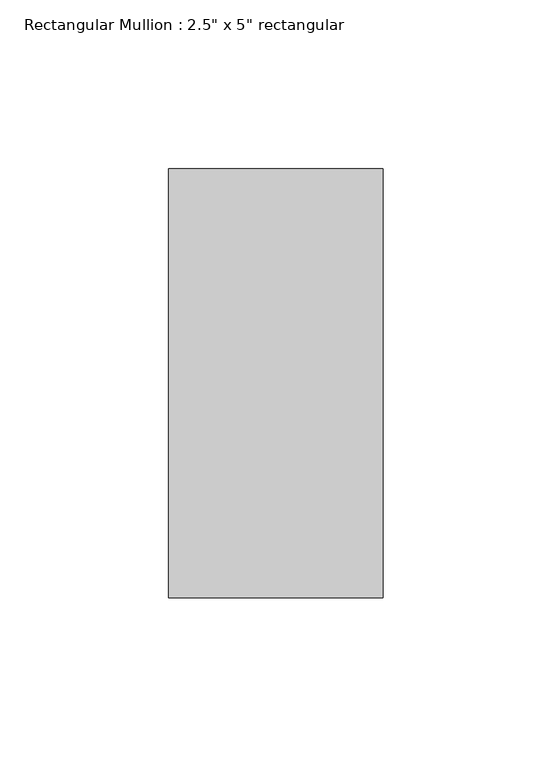
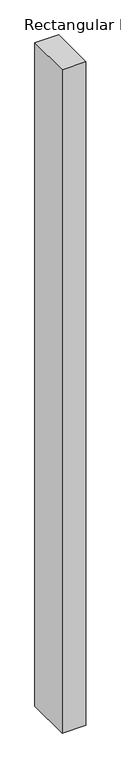
"""IFC4 building model written with IfcOpenShell, lengths in millimetres: member geometry."""

from ifc_helpers import new_model, si_unit, frame, origin, place, context, project, spatial, polyline, outline, extrude, source, transform, mapped, element, save


def member_6a6f69b9(model_context):
    return source(origin(), model_context, "Body", "SweptSolid", [
        extrude(outline(polyline([(31.75, 63.5), (31.75, -63.5), (-31.75, -63.5), (-31.75, 63.5), (31.75, 63.5)])), frame((0.0, 0.0, -1887.2910101), z_axis=(0.0, 0.0, 1.0), x_axis=(1.0, 0.0, 0.0)), (0.0, 0.0, 1.0), 1887.2910101),
    ])


if __name__ == "__main__":
    model = new_model("IFC4")
    model_context = context("Model", 3, world=origin())
    ifc_project = project(units=[si_unit("LENGTHUNIT", "METRE", prefix="MILLI")], contexts=[model_context])
    site = spatial("IfcSite", under=ifc_project)
    building = spatial("IfcBuilding", under=site)
    placement = place(None, origin())
    member_shape = member_6a6f69b9(model_context)
    element("IfcMember", 1, ObjectType="Rectangular Mullion : 2.5\" x 5\" rectangular", at=placement, inside=building, context=model_context, shape_type="MappedRepresentation", body=[
        mapped(member_shape, transform((0.0, 0.0, 0.0), x_axis=(1.0, 0.0, 0.0), y_axis=(0.0, 1.0, 0.0), z_axis=(0.0, 0.0, 1.0))),
    ])
    save(model, "model.ifc")

# Revit data of these elements
# Type "Rectangular Mullion : 2.5\" x 5\" rectangular"
#   built-in parameter 1007304 = 0.416667 (stored number, unit not read)
#   built-in parameter 1007301 = 0.104167 (stored number, unit not read)
#   built-in parameter 1007300 = 0.104167 (stored number, unit not read)
# Element 1 (IfcMember, "Rectangular Mullion : 2.5\" x 5\" rectangular")
#   Materials on its faces: "Aluminum"
# Materials
#   "Aluminum": class "Metal", colour RGB 247 247 247, transparency 0, Description = "Aluminum 6061", Cost = 0
